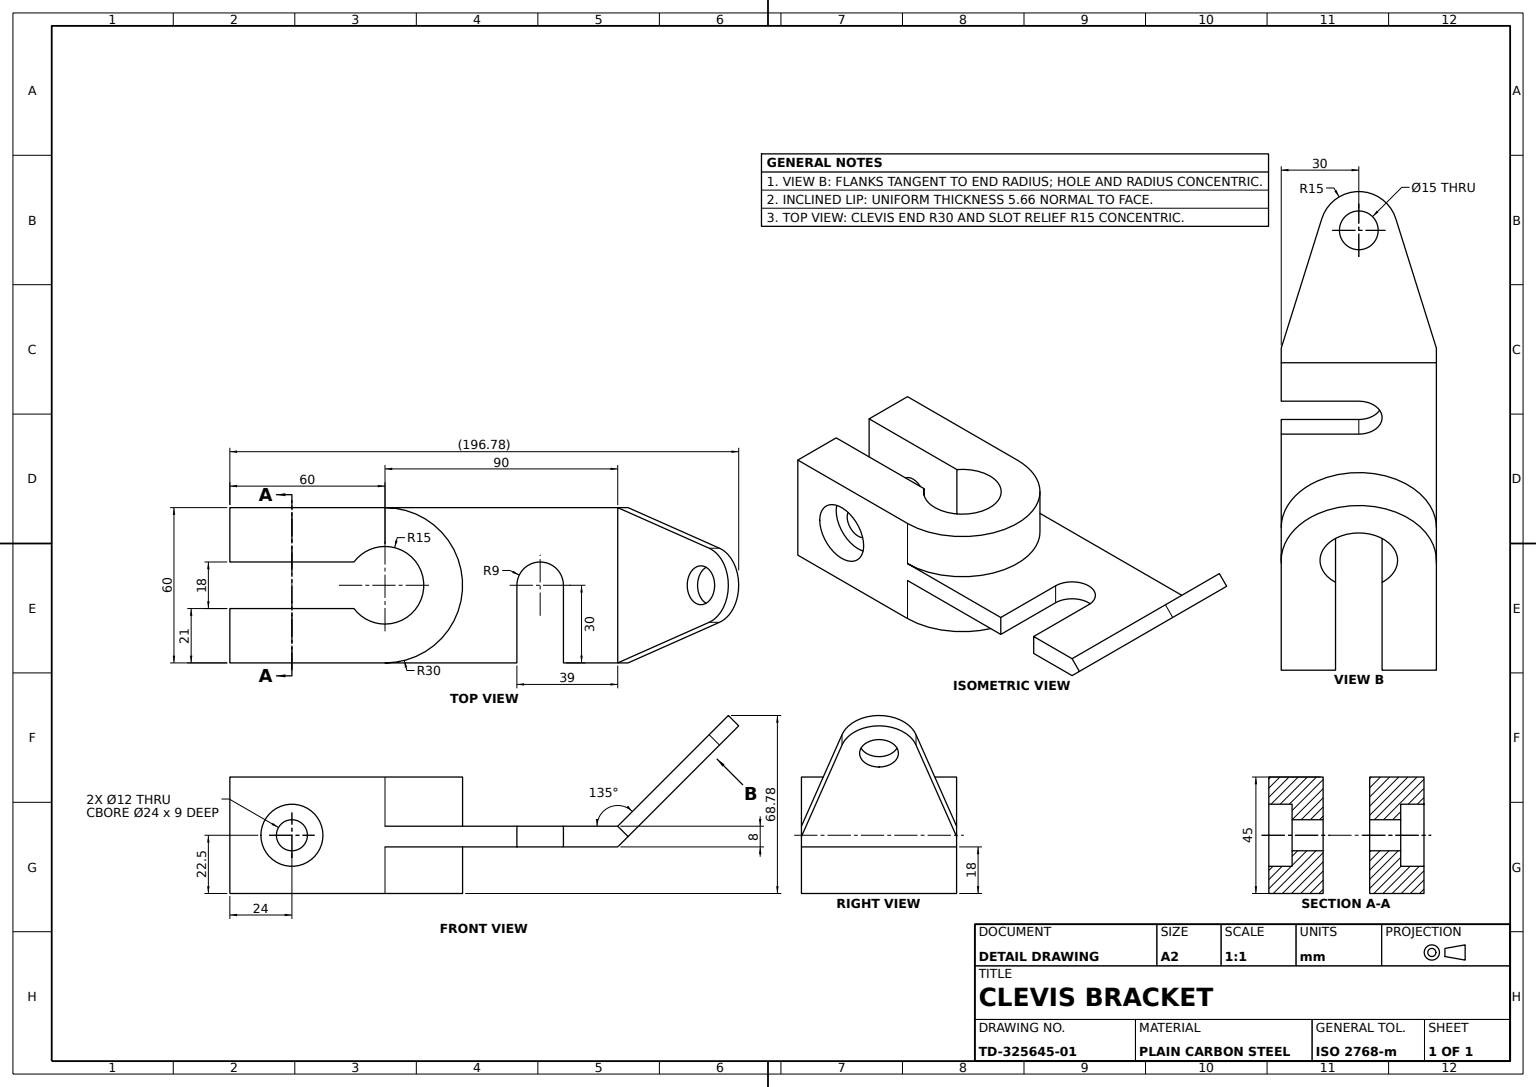
from build123d import *

# Parameters (mm, degrees)
BASE_BLOCK_DEPTH                       = 45
SLOTTED_TAB_DEPTH                      = 8
ANGLED_LIP_DEPTH                       = 60
CLEVIS_SLOT_DEPTH                      = 9
CLEVIS_CROSS_HOLE_M14_15_D             = 15
COUNTERBORED_BOLT_HOLE_M10_D           = 12
COUNTERBORED_BOLT_HOLE_M10_DEPTH       = 21
COUNTERBORED_BOLT_HOLE_M10_CBORE_D     = 24
COUNTERBORED_BOLT_HOLE_M10_CBORE_DEPTH = 9


with BuildPart() as part:
    # Base Block Sketch → Base Block (new body)
    with BuildSketch(Plane(origin=(0, 0, 0), x_dir=(1, 0, 0), z_dir=(0, 1, 0))):
        with BuildLine():
            Line((-60, 30), (-60, 9))
            Line((-60, 9), (-12, 9))
            ThreePointArc((-12, 9), (15, 0), (-12, -9))
            Line((-12, -9), (-60, -9))
            Line((-60, -9), (-60, -30))
            Line((-60, -30), (0, -30))
            ThreePointArc((0, -30), (30, 0), (0, 30))
            Line((0, 30), (-60, 30))
        make_face()
    extrude(amount=BASE_BLOCK_DEPTH)

    # Slotted Tab Sketch → Slotted Tab (add)
    with BuildSketch(Plane(origin=(0, 18, 0), x_dir=(-1, 0, 0), z_dir=(0, -1, 0))):
        with BuildLine():
            Line((0, 30), (-51, 30))
            Line((-51, 30), (-90, 30))
            Line((-90, 30), (-90, -30))
            Line((-90, -30), (-69, -30))
            Line((-69, -30), (-69, 0))
            ThreePointArc((-69, 0), (-60, 9), (-51, 0))
            Line((-51, 0), (-51, -30))
            Line((-51, -30), (0, -30))
            ThreePointArc((0, -30), (-30, 0), (0, 30))
        make_face()
    extrude(amount=-SLOTTED_TAB_DEPTH)

    # Angled Lip Sketch → Angled Lip (add)
    with BuildSketch(Plane.XY.offset(30)):
        Polygon((90, 18), (137, 65), (133, 69), (90, 26), align=None)
    extrude(amount=-ANGLED_LIP_DEPTH)

    # Clevis Slot Sketch → Clevis Slot (cut)
    with BuildSketch(Plane(origin=(32, -32, 0), x_dir=(0, 0, 1), z_dir=(-0.7071067811865439, 0.7071067811865512, 0))):
        with BuildLine():
            Line((-14.311818372, 132.015695434), (-30, 82.024386618))
            Line((-30, 82.024386618), (-33.812783533, 82.024386618))
            Line((-33.812783533, 82.024386618), (-33.812783533, 155.319200691))
            Line((-33.812783533, 155.319200691), (36.02403622, 155.319200691))
            Line((36.02403622, 155.319200691), (36.02403622, 82.024386618))
            Line((36.02403622, 82.024386618), (30, 82.024386618))
            Line((30, 82.024386618), (14.311818372, 132.015695434))
            ThreePointArc((14.311818372, 132.015695434), (0, 142.524386618), (-14.311818372, 132.015695434))
        make_face()
    extrude(amount=-CLEVIS_SLOT_DEPTH, mode=Mode.SUBTRACT)

    # Clevis Cross Hole M14 Ø15 (through all)
    with Locations(Plane(origin=(32, -32, 0), x_dir=(0.7071067811865512, 0.7071067811865439, 0), z_dir=(-0.7071067811865439, 0.7071067811865512, 0))):
        with Locations((127.524386618, 0)):
            Hole(CLEVIS_CROSS_HOLE_M14_15_D / 2)

    # Counterbored Bolt Hole M10
    with Locations(Plane.XY.offset(30)):
        with Locations((-36, 22.5)):
            counterbored_bolt_hole_m10 = CounterBoreHole(COUNTERBORED_BOLT_HOLE_M10_D / 2, COUNTERBORED_BOLT_HOLE_M10_CBORE_D / 2, COUNTERBORED_BOLT_HOLE_M10_CBORE_DEPTH, depth=COUNTERBORED_BOLT_HOLE_M10_DEPTH)

    # Bolt Hole Mirror: Counterbored Bolt Hole M10 across plane
    add(counterbored_bolt_hole_m10.mirror(Plane.XY), mode=Mode.SUBTRACT)


solid = part.part
